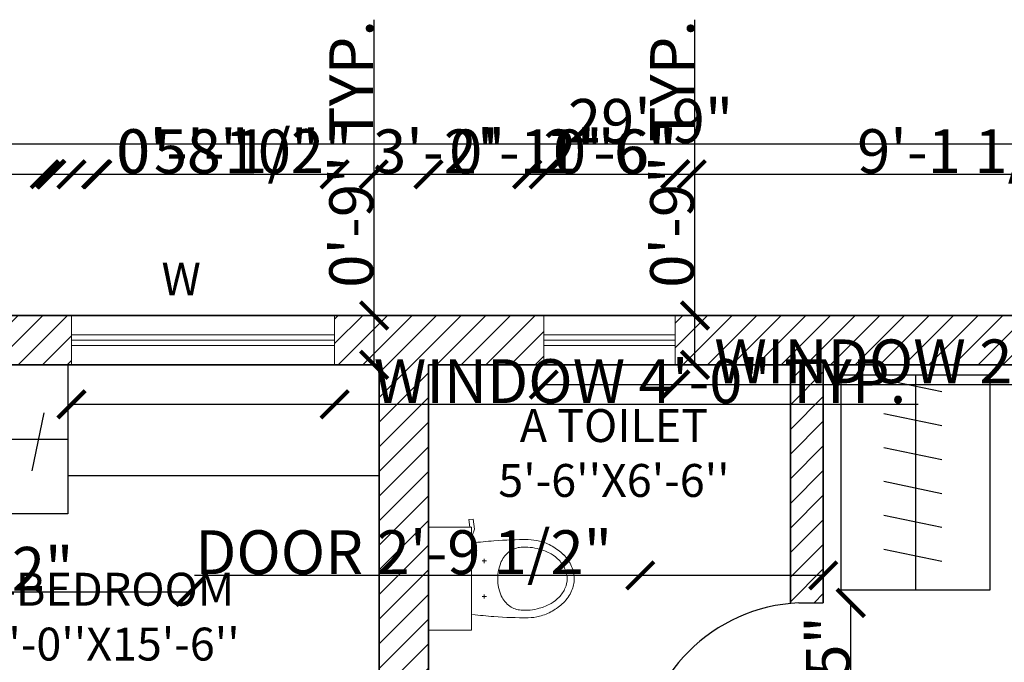
# Model space of a CAD drawing. Units: inches. Extents: x 2094 to 2639, y 1426 to 1997.
# Tile 7 of 8: x 2243 to 2423, y 1866 to 1983. Entities that reach past the tile are written whole.
import ezdxf

# ---------------------------------------------------------------- set-up
doc = ezdxf.new("R2010")
doc.units = ezdxf.units.IN
for name, color, linetype, lineweight in [('A-ANNO-DIMS', 2, 'Continuous', 18), ('A-ANNO-TEXT', 7, 'Continuous', 18), ('A-AREA-IDEN', 7, 'Continuous', 25), ('A-FLOR-CASE', 8, 'Continuous', 25), ('A-FLOR-FIXT', 9, 'Continuous', 18), ('A-WALL-PATT', 8, 'Continuous', 13), ('Doors', 34, 'Continuous', 25), ('Walls', 7, 'Continuous', 35), ('Windows', 150, 'Continuous', 18)]:
    doc.layers.add(name, color=color, linetype=linetype, lineweight=lineweight)
doc.styles.get("Standard").update_dxf_attribs({"font": 'arial.ttf'})
doc.dimstyles.get("Standard").update_dxf_attribs({"dimtxt": 8, "dimasz": 5, "dimexe": 0.18, "dimexo": 0.0625, "dimgap": 0.09, "dimtad": 1, "dimdec": 1, "dimzin": 0, "dimdsep": 46, "dimlunit": 4, "dimtxsty": 'Standard', "dimblk": 'ARCHTICK', "dimcen": 0.09, "dimse1": 1, "dimse2": 1, "dimadec": 0, "dimazin": 0, "dimtfac": 1, "dimtdec": 1, "dimtofl": 0, "dimtmove": 0, "dimatfit": 3, "dimfxl": 1, "dimtolj": 1, "dimtzin": 0, "dimarcsym": 0})

# ---------------------------------------------------------------- blocks, each defined once
blk = doc.blocks.new('AP0B05')
for p, q in [((35, 100), (35, 880)), ((75, 100), (75, 878.9)), ((35, 100), (35, -20)), ((815, 100), (815, -20))]:
    blk.add_line(p, q)
blk.add_lwpolyline([(35, 100), (75, 100)])
blk.add_arc((-2.4, 62.6), 818.3, 2.6212, 87.3788)
blk = doc.blocks.new('toilet-1')
at = {"color": 0, "linetype": 'ByBlock'}
for p, q in [((-0.23, -0.02), (-0.23, -0.2116)), ((0.23, -0.02), (-0.23, -0.02)), ((0.23, -0.02), (0.23, -0.2116)), ((-0.23, -0.2116), (0.23, -0.2116)), ((0.1917, -0.2144), (0.2206, -0.225)), ((0.2206, -0.225), (0.266, -0.2187)), ((0.2633, -0.1997), (0.23, -0.2044)), ((0.266, -0.2187), (0.2633, -0.1997)), ((-0.0793, -0.2587), (-0.0793, -0.2778)), ((0.0794, -0.2587), (0.0794, -0.2778)), ((-0.0889, -0.2683), (-0.0697, -0.2683)), ((0.0889, -0.2683), (0.0698, -0.2683)), ((0, -0.6382), (0, -0.6382))]:
    blk.add_line(p, q, dxfattribs=at)
for centre, radius, start, end in [((3.5272, -0.6239), 3.7093, 173.6925, 175.1593), ((-3.527, -0.624), 3.7093, 4.8413, 6.3171), ((1.7368, -0.4519), 1.9109, 175.7698, 180.3758), ((-0.0312, -0.4465), 0.1114, 113.8997, 145.1485), ((0, -0.5169), 0.1884, 66.0939, 113.9061), ((0.0312, -0.4465), 0.1114, 34.8515, 66.1003), ((-1.7366, -0.4519), 1.9109, 359.6242, 4.2302), ((-0.0408, -0.4398), 0.0996, 145.1497, 175.881), ((0.0409, -0.4398), 0.0996, 4.119, 34.8503), ((0.0981, -0.4497), 0.2389, 175.8862, 195.5931), ((-0.098, -0.4497), 0.2389, 344.4069, 4.1138), ((0.0353, -0.463), 0.2093, 180.3747, 194.3375), ((-0.0351, -0.463), 0.2093, 345.6614, 359.6243), ((0.055, -0.458), 0.2297, 194.3353, 209.622), ((0.0961, -0.4503), 0.2369, 195.5969, 209.3771), ((-0.096, -0.4503), 0.2369, 330.6229, 344.4031), ((-0.0548, -0.458), 0.2297, 330.3788, 345.6655), ((0.0232, -0.4913), 0.1532, 209.3871, 226.5438), ((-0.0231, -0.4913), 0.1532, 313.4562, 330.6129), ((0.0647, -0.4524), 0.2409, 209.6273, 224.5489), ((0.0152, -0.4997), 0.1416, 226.5501, 246.5527), ((-0.0151, -0.4997), 0.1416, 293.4473, 313.4499), ((-0.0645, -0.4524), 0.2409, 315.4504, 330.372), ((0.0178, -0.4986), 0.1751, 224.552, 245.714), ((0.0004, -0.538), 0.132, 245.5845, 269.8782), ((0, -0.5347), 0.1034, 246.5493, 270.0042), ((0, -0.5347), 0.1034, 269.9958, 293.4507), ((-0.0002, -0.538), 0.132, 270.1216, 294.4153), ((-0.0176, -0.4986), 0.1751, 294.2865, 315.4485)]:
    blk.add_arc(centre, radius, start, end, dxfattribs=at)
blk = doc.blocks.new('_ArchTick')
at = {"color": 0, "linetype": 'ByBlock', "const_width": 0.15}
blk.add_lwpolyline([(-0.5, -0.5), (0.5, 0.5)], dxfattribs=at)
blk = doc.blocks.new('*D13')
at = {"layer": 'A-ANNO-DIMS', "color": 0, "lineweight": -2, "transparency": 16777216}
blk.add_line((2180.06, 1960.22), (2537.06, 1960.22), dxfattribs=at)
at = {"layer": 'Defpoints', "color": 0, "transparency": 16777216}
for p in [(2537.06, 1960.22), (2180.06, 1928.9), (2537.06, 1928.9)]:
    blk.add_point(p, dxfattribs=at)
at = {"layer": 'A-ANNO-DIMS', "color": 0, "lineweight": -2, "transparency": 16777216, "xscale": 5, "yscale": 5, "zscale": 5, "rotation": 180}
blk.add_blockref('_ArchTick', (2180.06, 1960.22), dxfattribs=at)
at = {"layer": 'A-ANNO-DIMS', "color": 0, "lineweight": -2, "transparency": 16777216, "xscale": 5, "yscale": 5, "zscale": 5}
blk.add_blockref('_ArchTick', (2537.06, 1960.22), dxfattribs=at)
at = {"layer": 'A-ANNO-DIMS', "color": 0, "transparency": 16777216, "insert": (2358.56, 1964.39), "char_height": 8, "attachment_point": 5}
blk.add_mtext('\\A1;29\'-9"', dxfattribs=at)
blk = doc.blocks.new('WIN-48IN')
for p, q in [((0, 5.5), (48, 5.5)), ((0, 4.5), (48, 4.5)), ((0, 3.5), (48, 3.5))]:
    blk.add_line(p, q)
blk.add_lwpolyline([(0, 0), (48, 0), (48, 9), (0, 9)], close=True)
blk = doc.blocks.new('WIN-24IN')
for p, q in [((24, 5.5), (0, 5.5)), ((24, 4.5), (0, 4.5)), ((24, 3.5), (0, 3.5))]:
    blk.add_line(p, q)
blk.add_lwpolyline([(24, 9), (0, 9), (0, 0), (24, 0)], close=True)
blk = doc.blocks.new('*D19')
at = {"layer": 'A-ANNO-DIMS', "color": 0, "lineweight": -2, "transparency": 16777216}
for p, q in [((2356.68, 1881.5), (2275.36, 1881.5)), ((2390.06, 1881.5), (2356.68, 1881.5))]:
    blk.add_line(p, q, dxfattribs=at)
at = {"layer": 'Defpoints', "color": 0, "transparency": 16777216}
for p in [(2356.68, 1881.5), (2356.68, 1876.49), (2390.06, 1876.49)]:
    blk.add_point(p, dxfattribs=at)
at = {"layer": 'A-ANNO-DIMS', "color": 0, "lineweight": -2, "transparency": 16777216, "xscale": 5, "yscale": 5, "zscale": 5, "rotation": 180}
blk.add_blockref('_ArchTick', (2356.68, 1881.5), dxfattribs=at)
at = {"layer": 'A-ANNO-DIMS', "color": 0, "lineweight": -2, "transparency": 16777216, "xscale": 5, "yscale": 5, "zscale": 5}
blk.add_blockref('_ArchTick', (2390.06, 1881.5), dxfattribs=at)
at = {"layer": 'A-ANNO-DIMS', "color": 0, "transparency": 16777216, "insert": (2313.52, 1885.73), "char_height": 8, "attachment_point": 5}
blk.add_mtext('\\A1;DOOR 2\'-9 1/2"', dxfattribs=at)
blk = doc.blocks.new('*D20')
at = {"layer": 'A-ANNO-DIMS', "color": 0, "lineweight": -2, "transparency": 16777216}
blk.add_line((2395.06, 1847.57), (2395.06, 1876.49), dxfattribs=at)
at = {"layer": 'Defpoints', "color": 0, "transparency": 16777216}
for p in [(2390.06, 1876.49), (2395.06, 1876.49), (2390.06, 1847.57)]:
    blk.add_point(p, dxfattribs=at)
at = {"layer": 'A-ANNO-DIMS', "color": 0, "lineweight": -2, "transparency": 16777216, "xscale": 5, "yscale": 5, "zscale": 5}
for p, rotation in [((2395.06, 1876.49), 90), ((2395.06, 1847.57), 270)]:
    blk.add_blockref('_ArchTick', p, dxfattribs=dict(at, rotation=rotation))
at = {"layer": 'A-ANNO-DIMS', "color": 0, "transparency": 16777216, "insert": (2390.89, 1862.03), "char_height": 8, "attachment_point": 5, "rotation": 90}
blk.add_mtext('\\A1;2\'-5"', dxfattribs=at)
blk = doc.blocks.new('*D27')
at = {"layer": 'A-ANNO-DIMS', "color": 0, "lineweight": -2, "transparency": 16777216}
for p, q in [((2252.94, 1912.7), (2300.94, 1912.7)), ((2300.94, 1912.7), (2407.35, 1912.7))]:
    blk.add_line(p, q, dxfattribs=at)
at = {"layer": 'Defpoints', "color": 0, "transparency": 16777216}
for p in [(2252.94, 1919.9), (2300.94, 1919.9), (2300.94, 1912.7)]:
    blk.add_point(p, dxfattribs=at)
at = {"layer": 'A-ANNO-DIMS', "color": 0, "lineweight": -2, "transparency": 16777216, "xscale": 5, "yscale": 5, "zscale": 5, "rotation": 180}
blk.add_blockref('_ArchTick', (2252.94, 1912.7), dxfattribs=at)
at = {"layer": 'A-ANNO-DIMS', "color": 0, "lineweight": -2, "transparency": 16777216, "xscale": 5, "yscale": 5, "zscale": 5}
blk.add_blockref('_ArchTick', (2300.94, 1912.7), dxfattribs=at)
at = {"layer": 'A-ANNO-DIMS', "color": 0, "transparency": 16777216, "insert": (2356.64, 1916.93), "char_height": 8, "attachment_point": 5}
blk.add_mtext('\\A1;WINDOW 4\'-0" TYP.', dxfattribs=at)
blk = doc.blocks.new('*D28')
at = {"layer": 'A-ANNO-DIMS', "color": 0, "lineweight": -2, "transparency": 16777216}
for p, q in [((2308.14, 1928.9), (2308.14, 1982.84)), ((2308.14, 1919.9), (2308.14, 1928.9))]:
    blk.add_line(p, q, dxfattribs=at)
at = {"layer": 'Defpoints', "color": 0, "transparency": 16777216}
for p in [(2300.94, 1928.9), (2308.14, 1928.9), (2300.94, 1919.9)]:
    blk.add_point(p, dxfattribs=at)
at = {"layer": 'A-ANNO-DIMS', "color": 0, "lineweight": -2, "transparency": 16777216, "xscale": 5, "yscale": 5, "zscale": 5}
for p, rotation in [((2308.14, 1928.9), 90), ((2308.14, 1919.9), 270)]:
    blk.add_blockref('_ArchTick', p, dxfattribs=dict(at, rotation=rotation))
at = {"layer": 'A-ANNO-DIMS', "color": 0, "transparency": 16777216, "insert": (2303.96, 1958.37), "char_height": 8, "attachment_point": 5, "rotation": 90}
blk.add_mtext('\\A1;0\'-9" TYP.', dxfattribs=at)
blk = doc.blocks.new('*D29')
at = {"layer": 'A-ANNO-DIMS', "color": 0, "lineweight": -2, "transparency": 16777216}
for p, q in [((2339.06, 1916.3), (2363.06, 1916.3)), ((2363.06, 1916.3), (2469.47, 1916.3))]:
    blk.add_line(p, q, dxfattribs=at)
at = {"layer": 'Defpoints', "color": 0, "transparency": 16777216}
for p in [(2339.06, 1919.9), (2363.06, 1919.9), (2363.06, 1916.3)]:
    blk.add_point(p, dxfattribs=at)
at = {"layer": 'A-ANNO-DIMS', "color": 0, "lineweight": -2, "transparency": 16777216, "xscale": 5, "yscale": 5, "zscale": 5, "rotation": 180}
blk.add_blockref('_ArchTick', (2339.06, 1916.3), dxfattribs=at)
at = {"layer": 'A-ANNO-DIMS', "color": 0, "lineweight": -2, "transparency": 16777216, "xscale": 5, "yscale": 5, "zscale": 5}
blk.add_blockref('_ArchTick', (2363.06, 1916.3), dxfattribs=at)
at = {"layer": 'A-ANNO-DIMS', "color": 0, "transparency": 16777216, "insert": (2418.76, 1920.53), "char_height": 8, "attachment_point": 5}
blk.add_mtext('\\A1;WINDOW 2\'-0" TYP.', dxfattribs=at)
blk = doc.blocks.new('*D30')
at = {"layer": 'A-ANNO-DIMS', "color": 0, "lineweight": -2, "transparency": 16777216}
for p, q in [((2366.66, 1928.9), (2366.66, 1982.84)), ((2366.66, 1919.9), (2366.66, 1928.9))]:
    blk.add_line(p, q, dxfattribs=at)
at = {"layer": 'Defpoints', "color": 0, "transparency": 16777216}
for p in [(2363.06, 1928.9), (2366.66, 1928.9), (2363.06, 1919.9)]:
    blk.add_point(p, dxfattribs=at)
at = {"layer": 'A-ANNO-DIMS', "color": 0, "lineweight": -2, "transparency": 16777216, "xscale": 5, "yscale": 5, "zscale": 5}
for p, rotation in [((2366.66, 1928.9), 90), ((2366.66, 1919.9), 270)]:
    blk.add_blockref('_ArchTick', p, dxfattribs=dict(at, rotation=rotation))
at = {"layer": 'A-ANNO-DIMS', "color": 0, "transparency": 16777216, "insert": (2362.48, 1958.37), "char_height": 8, "attachment_point": 5, "rotation": 90}
blk.add_mtext('\\A1;0\'-9" TYP.', dxfattribs=at)
blk = doc.blocks.new('*D34')
at = {"layer": 'A-ANNO-DIMS', "color": 0, "lineweight": -2, "transparency": 16777216}
blk.add_line((2274.56, 1878.47), (2189.06, 1878.47), dxfattribs=at)
at = {"layer": 'Defpoints', "color": 0, "transparency": 16777216}
for p in [(2189.06, 1878.47), (2189.06, 1862.67), (2274.56, 1862.67)]:
    blk.add_point(p, dxfattribs=at)
at = {"layer": 'A-ANNO-DIMS', "color": 0, "lineweight": -2, "transparency": 16777216, "xscale": 5, "yscale": 5, "zscale": 5, "rotation": 180}
blk.add_blockref('_ArchTick', (2189.06, 1878.47), dxfattribs=at)
at = {"layer": 'A-ANNO-DIMS', "color": 0, "lineweight": -2, "transparency": 16777216, "xscale": 5, "yscale": 5, "zscale": 5}
blk.add_blockref('_ArchTick', (2274.56, 1878.47), dxfattribs=at)
at = {"layer": 'A-ANNO-DIMS', "color": 0, "transparency": 16777216, "insert": (2231.81, 1882.7), "char_height": 8, "attachment_point": 5}
blk.add_mtext('\\A1;7\'-1 1/2"', dxfattribs=at)
blk = doc.blocks.new('*D53')
at = {"layer": 'A-ANNO-DIMS', "color": 0, "lineweight": -2, "transparency": 16777216}
blk.add_line((2180.06, 1954.65), (2252.94, 1954.65), dxfattribs=at)
at = {"layer": 'Defpoints', "color": 0, "transparency": 16777216}
for p in [(2252.94, 1954.65), (2180.06, 1928.9), (2252.94, 1928.9)]:
    blk.add_point(p, dxfattribs=at)
at = {"layer": 'A-ANNO-DIMS', "color": 0, "lineweight": -2, "transparency": 16777216, "xscale": 5, "yscale": 5, "zscale": 5, "rotation": 180}
blk.add_blockref('_ArchTick', (2180.06, 1954.65), dxfattribs=at)
at = {"layer": 'A-ANNO-DIMS', "color": 0, "lineweight": -2, "transparency": 16777216, "xscale": 5, "yscale": 5, "zscale": 5}
blk.add_blockref('_ArchTick', (2252.94, 1954.65), dxfattribs=at)
at = {"layer": 'A-ANNO-DIMS', "color": 0, "transparency": 16777216, "insert": (2216.5, 1958.82), "char_height": 8, "attachment_point": 5}
blk.add_mtext('\\A1;6\'-1"', dxfattribs=at)
blk = doc.blocks.new('*D54')
at = {"layer": 'A-ANNO-DIMS', "color": 0, "lineweight": -2, "transparency": 16777216}
blk.add_line((2300.94, 1954.65), (2339.06, 1954.65), dxfattribs=at)
at = {"layer": 'Defpoints', "color": 0, "transparency": 16777216}
for p in [(2339.06, 1954.65), (2300.94, 1928.9), (2339.06, 1928.9)]:
    blk.add_point(p, dxfattribs=at)
at = {"layer": 'A-ANNO-DIMS', "color": 0, "lineweight": -2, "transparency": 16777216, "xscale": 5, "yscale": 5, "zscale": 5, "rotation": 180}
blk.add_blockref('_ArchTick', (2300.94, 1954.65), dxfattribs=at)
at = {"layer": 'A-ANNO-DIMS', "color": 0, "lineweight": -2, "transparency": 16777216, "xscale": 5, "yscale": 5, "zscale": 5}
blk.add_blockref('_ArchTick', (2339.06, 1954.65), dxfattribs=at)
at = {"layer": 'A-ANNO-DIMS', "color": 0, "transparency": 16777216, "insert": (2320, 1958.83), "char_height": 8, "attachment_point": 5}
blk.add_mtext('\\A1;3\'-2"', dxfattribs=at)
blk = doc.blocks.new('*D55')
at = {"layer": 'A-ANNO-DIMS', "color": 0, "lineweight": -2, "transparency": 16777216}
blk.add_line((2363.06, 1954.65), (2472.33, 1954.65), dxfattribs=at)
at = {"layer": 'Defpoints', "color": 0, "transparency": 16777216}
for p in [(2472.33, 1954.65), (2363.06, 1928.9), (2472.33, 1928.9)]:
    blk.add_point(p, dxfattribs=at)
at = {"layer": 'A-ANNO-DIMS', "color": 0, "lineweight": -2, "transparency": 16777216, "xscale": 5, "yscale": 5, "zscale": 5, "rotation": 180}
blk.add_blockref('_ArchTick', (2363.06, 1954.65), dxfattribs=at)
at = {"layer": 'A-ANNO-DIMS', "color": 0, "lineweight": -2, "transparency": 16777216, "xscale": 5, "yscale": 5, "zscale": 5}
blk.add_blockref('_ArchTick', (2472.33, 1954.65), dxfattribs=at)
at = {"layer": 'A-ANNO-DIMS', "color": 0, "transparency": 16777216, "insert": (2417.69, 1958.87), "char_height": 8, "attachment_point": 5}
blk.add_mtext('\\A1;9\'-1 1/2"', dxfattribs=at)
blk = doc.blocks.new('*D66')
at = {"layer": 'A-ANNO-DIMS', "color": 0, "lineweight": -2, "transparency": 16777216}
blk.add_line((2336.06, 1954.65), (2366.06, 1954.65), dxfattribs=at)
at = {"layer": 'Defpoints', "color": 0, "transparency": 16777216}
for p in [(2366.06, 1954.65), (2336.06, 1787.9), (2366.06, 1787.9)]:
    blk.add_point(p, dxfattribs=at)
at = {"layer": 'A-ANNO-DIMS', "color": 0, "lineweight": -2, "transparency": 16777216, "xscale": 5, "yscale": 5, "zscale": 5, "rotation": 180}
blk.add_blockref('_ArchTick', (2336.06, 1954.65), dxfattribs=at)
at = {"layer": 'A-ANNO-DIMS', "color": 0, "lineweight": -2, "transparency": 16777216, "xscale": 5, "yscale": 5, "zscale": 5}
blk.add_blockref('_ArchTick', (2366.06, 1954.65), dxfattribs=at)
at = {"layer": 'A-ANNO-DIMS', "color": 0, "transparency": 16777216, "insert": (2351.06, 1958.82), "char_height": 8, "attachment_point": 5}
blk.add_mtext('\\A1;2\'-6"', dxfattribs=at)
blk = doc.blocks.new('*D76')
at = {"layer": 'A-ANNO-DIMS', "color": 0, "lineweight": -2, "transparency": 16777216}
blk.add_line((2248.06, 1954.65), (2318.06, 1954.65), dxfattribs=at)
at = {"layer": 'Defpoints', "color": 0, "transparency": 16777216}
for p in [(2318.06, 1954.65), (2248.06, 1468.9), (2318.06, 1468.9)]:
    blk.add_point(p, dxfattribs=at)
at = {"layer": 'A-ANNO-DIMS', "color": 0, "lineweight": -2, "transparency": 16777216, "xscale": 5, "yscale": 5, "zscale": 5, "rotation": 180}
blk.add_blockref('_ArchTick', (2248.06, 1954.65), dxfattribs=at)
at = {"layer": 'A-ANNO-DIMS', "color": 0, "lineweight": -2, "transparency": 16777216, "xscale": 5, "yscale": 5, "zscale": 5}
blk.add_blockref('_ArchTick', (2318.06, 1954.65), dxfattribs=at)
at = {"layer": 'A-ANNO-DIMS', "color": 0, "transparency": 16777216, "insert": (2283.06, 1958.82), "char_height": 8, "attachment_point": 5}
blk.add_mtext('\\A1;5\'-10"', dxfattribs=at)
blk = doc.blocks.new('*D77')
at = {"layer": 'A-ANNO-DIMS', "color": 0, "lineweight": -2, "transparency": 16777216}
for p, q in [((2308.06, 1954.65), (2318.06, 1954.65)), ((2318.06, 1954.65), (2350.72, 1954.65))]:
    blk.add_line(p, q, dxfattribs=at)
at = {"layer": 'Defpoints', "color": 0, "transparency": 16777216}
for p in [(2318.06, 1954.65), (2308.06, 1468.9), (2318.06, 1468.9)]:
    blk.add_point(p, dxfattribs=at)
at = {"layer": 'A-ANNO-DIMS', "color": 0, "lineweight": -2, "transparency": 16777216, "xscale": 5, "yscale": 5, "zscale": 5, "rotation": 180}
blk.add_blockref('_ArchTick', (2308.06, 1954.65), dxfattribs=at)
at = {"layer": 'A-ANNO-DIMS', "color": 0, "lineweight": -2, "transparency": 16777216, "xscale": 5, "yscale": 5, "zscale": 5}
blk.add_blockref('_ArchTick', (2318.06, 1954.65), dxfattribs=at)
at = {"layer": 'A-ANNO-DIMS', "color": 0, "transparency": 16777216, "insert": (2336.89, 1958.82), "char_height": 8, "attachment_point": 5}
blk.add_mtext('\\A1;0\'-10"', dxfattribs=at)
blk = doc.blocks.new('*D80')
at = {"layer": 'A-ANNO-DIMS', "color": 0, "lineweight": -2, "transparency": 16777216}
for p, q in [((2318.06, 1954.65), (2336.06, 1954.65)), ((2336.06, 1954.65), (2361.75, 1954.65))]:
    blk.add_line(p, q, dxfattribs=at)
at = {"layer": 'Defpoints', "color": 0, "transparency": 16777216}
for p in [(2336.06, 1954.65), (2318.06, 1787.9), (2336.06, 1787.9)]:
    blk.add_point(p, dxfattribs=at)
at = {"layer": 'A-ANNO-DIMS', "color": 0, "lineweight": -2, "transparency": 16777216, "xscale": 5, "yscale": 5, "zscale": 5, "rotation": 180}
blk.add_blockref('_ArchTick', (2318.06, 1954.65), dxfattribs=at)
at = {"layer": 'A-ANNO-DIMS', "color": 0, "lineweight": -2, "transparency": 16777216, "xscale": 5, "yscale": 5, "zscale": 5}
blk.add_blockref('_ArchTick', (2336.06, 1954.65), dxfattribs=at)
at = {"layer": 'A-ANNO-DIMS', "color": 0, "transparency": 16777216, "insert": (2351.4, 1958.82), "char_height": 8, "attachment_point": 5}
blk.add_mtext('\\A1;1\'-6"', dxfattribs=at)
blk = doc.blocks.new('*D81')
at = {"layer": 'A-ANNO-DIMS', "color": 0, "lineweight": -2, "transparency": 16777216}
for p, q in [((2249.13, 1954.65), (2257.66, 1954.65)), ((2257.66, 1954.65), (2302.74, 1954.65))]:
    blk.add_line(p, q, dxfattribs=at)
at = {"layer": 'Defpoints', "color": 0, "transparency": 16777216}
for p in [(2257.66, 1954.65), (2249.13, 1589.48), (2257.66, 1589.48)]:
    blk.add_point(p, dxfattribs=at)
at = {"layer": 'A-ANNO-DIMS', "color": 0, "lineweight": -2, "transparency": 16777216, "xscale": 5, "yscale": 5, "zscale": 5, "rotation": 180}
blk.add_blockref('_ArchTick', (2249.13, 1954.65), dxfattribs=at)
at = {"layer": 'A-ANNO-DIMS', "color": 0, "lineweight": -2, "transparency": 16777216, "xscale": 5, "yscale": 5, "zscale": 5}
blk.add_blockref('_ArchTick', (2257.66, 1954.65), dxfattribs=at)
at = {"layer": 'A-ANNO-DIMS', "color": 0, "transparency": 16777216, "insert": (2282.7, 1958.87), "char_height": 8, "attachment_point": 5}
blk.add_mtext('\\A1;0\'-8 1/2"', dxfattribs=at)
blk = doc.blocks.new('*D83')
at = {"layer": 'A-ANNO-DIMS', "color": 0, "lineweight": -2, "transparency": 16777216}
for p, q in [((2249.25, 1954.65), (2257.43, 1954.65)), ((2257.43, 1954.65), (2283.88, 1954.65))]:
    blk.add_line(p, q, dxfattribs=at)
at = {"layer": 'Defpoints', "color": 0, "transparency": 16777216}
for p in [(2257.43, 1954.65), (2249.25, 1595.79), (2257.43, 1595.79)]:
    blk.add_point(p, dxfattribs=at)
at = {"layer": 'A-ANNO-DIMS', "color": 0, "lineweight": -2, "transparency": 16777216, "xscale": 5, "yscale": 5, "zscale": 5, "rotation": 180}
blk.add_blockref('_ArchTick', (2249.25, 1954.65), dxfattribs=at)
at = {"layer": 'A-ANNO-DIMS', "color": 0, "lineweight": -2, "transparency": 16777216, "xscale": 5, "yscale": 5, "zscale": 5}
blk.add_blockref('_ArchTick', (2257.43, 1954.65), dxfattribs=at)
at = {"layer": 'A-ANNO-DIMS', "color": 0, "transparency": 16777216, "insert": (2273.16, 1958.82), "char_height": 8, "attachment_point": 5}
blk.add_mtext('\\A1;0\'-8"', dxfattribs=at)

msp = doc.modelspace()

# ---------------------------------------------------------------- hatches: boundary and pattern name
at = {"layer": 'A-WALL-PATT', "transparency": 33554585}
h = msp.add_hatch(dxfattribs=at)
h.set_pattern_fill('ANSI31', color=256)
h.paths.add_polyline_path([(2189.06, 1727.9), (2230.3, 1727.9, -0.022928), (2230.09, 1730.2), (2230.09, 1733.9), (2189.06, 1733.9), (2189.06, 1742.37), (2180.06, 1742.37), (2180.06, 1714.4), (2189.06, 1714.4)])
h.paths.add_polyline_path([(2456.51, 1574.9), (2413.83, 1574.9), (2413.83, 1565.9), (2456.51, 1565.9)])
h.paths.add_polyline_path([(2537.06, 1643.81), (2528.06, 1643.81), (2528.06, 1574.9), (2519.78, 1574.9), (2519.78, 1571.88), (2519.78, 1565.9), (2537.06, 1565.9)])
h.paths.add_polyline_path([(2339.06, 1928.9), (2300.94, 1928.9), (2300.94, 1919.9), (2309.06, 1919.9), (2309.06, 1776.3, -0.024186), (2312.62, 1776.64), (2318.06, 1776.64), (2318.06, 1778.9), (2336.06, 1778.9), (2336.06, 1787.9), (2318.06, 1787.9), (2318.06, 1835.9), (2384.06, 1835.9), (2384.06, 1787.9), (2366.06, 1787.9), (2366.06, 1778.9), (2479.64, 1778.9), (2479.64, 1784.88, -0.018603), (2479.89, 1787.9), (2390.06, 1787.9), (2390.06, 1847.57), (2385.61, 1847.57), (2384.06, 1847.57), (2384.06, 1841.9), (2318.06, 1841.9), (2318.06, 1919.9), (2339.06, 1919.9)])
h.paths.add_polyline_path([(2252.94, 1928.9), (2180.06, 1928.9), (2180.06, 1790.37), (2189.06, 1790.37), (2189.06, 1843.77), (2189.06, 1919.9), (2252.94, 1919.9)])
h.paths.add_polyline_path([(2472.33, 1928.9), (2363.06, 1928.9), (2363.06, 1919.9), (2384.06, 1919.9), (2384.06, 1876.38, -0.012802), (2385.61, 1876.49), (2390.06, 1876.49), (2390.06, 1919.9), (2472.33, 1919.9)], flags=17)
h.paths.add_polyline_path([(2537.06, 1928.9), (2520.33, 1928.9), (2520.33, 1919.9), (2528.06, 1919.9), (2528.06, 1905.95), (2528.06, 1787.9), (2518.5, 1787.9), (2518.5, 1784.88), (2518.5, 1778.9), (2528.06, 1778.9), (2528.06, 1715.81), (2537.06, 1715.81)])
h.paths.add_polyline_path([(2379.33, 1857.12), (2393.06, 1857.12), (2393.06, 1866.16), (2379.33, 1866.16)], flags=25)
h.paths.add_polyline_path([(2235.85, 1725.77), (2249.57, 1725.77), (2249.57, 1734.81), (2235.85, 1734.81)], flags=25)
h.paths.add_polyline_path([(2305.79, 1754.6), (2314.84, 1754.6), (2314.84, 1763.6), (2305.79, 1763.6)], flags=9)
h.paths.add_polyline_path([(2493.85, 1778.22), (2502.9, 1778.22), (2502.9, 1787.22), (2493.85, 1787.22)], flags=9)
h.paths.add_polyline_path([(2370.69, 1555.65), (2381.6, 1555.65), (2381.6, 1564.65), (2370.69, 1564.65)], flags=9)
h.paths.add_polyline_path([(2461.57, 1555.65), (2477.6, 1555.65), (2477.6, 1564.65), (2461.57, 1564.65)], flags=9)
h.paths.add_polyline_path([(2493.18, 1565.15), (2509.22, 1565.15), (2509.22, 1574.15), (2493.18, 1574.15)], flags=9)
h.paths.add_polyline_path([(2408.32, 1501.7), (2449.12, 1501.7), (2449.12, 1520.36), (2408.32, 1520.36)], flags=9)
h.paths.add_polyline_path([(2398.49, 1698.6), (2441.61, 1698.6), (2441.61, 1717.26), (2398.49, 1717.26)], flags=9)
h.paths.add_polyline_path([(2248.63, 1683.29), (2287.87, 1683.29), (2287.87, 1701.95), (2248.63, 1701.95)], flags=25)
h.paths.add_polyline_path([(2440.73, 1823.2), (2483.86, 1823.2), (2483.86, 1841.85), (2440.73, 1841.85)], flags=9)
h.paths.add_polyline_path([(2335.3, 1804.5), (2370.65, 1804.5), (2370.65, 1823.15), (2335.3, 1823.15)], flags=25)
h.paths.add_polyline_path([(2335.3, 1893.12), (2370.65, 1893.12), (2370.65, 1911.77), (2335.3, 1911.77)], flags=25)
h.paths.add_polyline_path([(2241.82, 1863.6), (2290.11, 1863.6), (2290.11, 1882.25), (2241.82, 1882.25)], flags=9)

# ---------------------------------------------------------------- linework, layer by layer
at = {"layer": 'A-FLOR-CASE'}
for p, q in [((2406.88, 1918.1), (2406.88, 1878.83)), ((2411.68, 1914.96), (2401.12, 1917.16)), ((2247.88, 1911.13), (2245.68, 1900.57)), ((2411.68, 1908.77), (2401.12, 1910.97)), ((2189.06, 1906.33), (2252.26, 1906.33)), ((2411.68, 1902.58), (2401.12, 1904.78)), ((2252.26, 1899.71), (2309.06, 1899.71)), ((2411.68, 1896.39), (2401.12, 1898.6)), ((2411.68, 1890.21), (2401.12, 1892.41)), ((2411.68, 1884.02), (2401.12, 1886.22))]:
    msp.add_line(p, q, dxfattribs=at)
for points in [[(2189.06, 1919.9), (2252.26, 1919.9), (2252.26, 1892.76), (2189.06, 1892.76)], [(2420.45, 1918.1), (2420.45, 1878.83), (2393.31, 1878.83), (2393.31, 1918.1)]]:
    msp.add_lwpolyline(points, close=True, dxfattribs=at)
at = {"layer": 'Walls'}
for p, q in [((2180.06, 1928.9), (2537.06, 1928.9)), ((2189.06, 1919.9), (2309.06, 1919.9)), ((2309.06, 1919.9), (2309.06, 1776.3)), ((2318.06, 1919.9), (2318.06, 1841.9)), ((2318.06, 1919.9), (2384.06, 1919.9)), ((2384.06, 1919.9), (2384.06, 1876.38)), ((2390.06, 1919.9), (2390.06, 1876.49)), ((2390.06, 1919.9), (2528.06, 1919.9))]:
    msp.add_line(p, q, dxfattribs=at)

# ---------------------------------------------------------------- block references
at = {"layer": 'A-FLOR-FIXT', "xscale": 40.90426662806183, "yscale": 40.90426662806183, "zscale": 40.90426662806183, "rotation": 90}
msp.add_blockref('toilet-1', (2317.24, 1880.9), dxfattribs=at)
at = {"layer": 'Doors', "xscale": 0.0370855999522285, "yscale": 0.0370855999522285, "zscale": 0.0370855999522285, "rotation": 90}
msp.add_blockref('AP0B05', (2389.31, 1846.27), dxfattribs=at)
at = {"layer": 'Windows'}
for name, p in [('WIN-48IN', (2252.94, 1919.9)), ('WIN-24IN', (2339.06, 1919.9))]:
    msp.add_blockref(name, p, dxfattribs=at)

# ---------------------------------------------------------------- texts
at = {"layer": 'A-ANNO-TEXT'}
msp.add_text('W', height=6, dxfattribs=at).set_placement((2269.35, 1932.56))
at = {"layer": 'A-AREA-IDEN', "char_height": 6, "attachment_point": 1}
for s, insert in [("\\pxqc;A TOILET\\P5'-6''X6'-6''", (2325.33, 1911.82)), ("\\pxqc;M-BEDROOM\\P10'-0''X15'-6''", (2231.43, 1881.98))]:
    msp.add_mtext_dynamic_manual_height_columns(s, width=53.0999, gutter_width=63.55, heights=[0], dxfattribs=dict(at, insert=insert))

# ---------------------------------------------------------------- dimensions: what is measured, and where the dimension line sits
at = {"layer": 'A-ANNO-DIMS'}
for base, p1, p2, angle, text, picture, middle in [((2308.14, 1928.9), (2300.94, 1919.9), (2300.94, 1928.9), 90, '<> TYP.', '*D28', (2303.96, 1958.37)), ((2366.66, 1928.9), (2363.06, 1919.9), (2363.06, 1928.9), 90, '<> TYP.', '*D30', (2362.48, 1958.37)), ((2356.68, 1881.5), (2390.06, 1876.49), (2356.68, 1876.49), 180, 'DOOR <>', '*D19', (2313.52, 1885.73))]:
    dim = msp.add_linear_dim(base=base, p1=p1, p2=p2, angle=angle, text=text, dimstyle='Standard', override={"dimdec": 1, "dimlfac": 1, "dimrnd": 0, "dimzin": 1, "dimdsep": 46, "dimlunit": 4, "dimfrac": 2}, dxfattribs=at)
    dim.commit()
    dim.dimension.update_dxf_attribs({"geometry": picture, "text_midpoint": middle})
for base, p1, p2, override, picture, middle in [((2257.66, 1954.65), (2249.13, 1589.48), (2257.66, 1589.48), {"dimdec": 1, "dimlfac": 1, "dimrnd": 0, "dimzin": 1, "dimdsep": 46, "dimlunit": 4, "dimfrac": 2}, '*D81', (2282.7, 1958.87)), ((2472.33, 1954.65), (2363.06, 1928.9), (2472.33, 1928.9), {"dimdec": 1, "dimlfac": 1, "dimrnd": 0, "dimzin": 1, "dimdsep": 46, "dimlunit": 4, "dimfrac": 2}, '*D55', (2417.69, 1958.87)), ((2537.06, 1960.22), (2180.06, 1928.9), (2537.06, 1928.9), {"dimclrd": 0, "dimclre": 0, "dimclrt": 0}, '*D13', (2358.56, 1964.39)), ((2252.94, 1954.65), (2180.06, 1928.9), (2252.94, 1928.9), {"dimdec": 1, "dimlfac": 1, "dimrnd": 0, "dimzin": 1, "dimdsep": 46, "dimlunit": 4, "dimfrac": 2}, '*D53', (2216.5, 1958.82)), ((2318.06, 1954.65), (2248.06, 1468.9), (2318.06, 1468.9), {"dimdec": 1, "dimlfac": 1, "dimrnd": 0, "dimzin": 1, "dimdsep": 46, "dimlunit": 4, "dimfrac": 2}, '*D76', (2283.06, 1958.82)), ((2257.43, 1954.65), (2249.25, 1595.79), (2257.43, 1595.79), {"dimdec": 1, "dimlfac": 1, "dimrnd": 0, "dimzin": 1, "dimdsep": 46, "dimlunit": 4, "dimfrac": 2}, '*D83', (2273.16, 1958.82)), ((2339.06, 1954.65), (2300.94, 1928.9), (2339.06, 1928.9), {"dimdec": 1, "dimlfac": 1, "dimrnd": 0, "dimzin": 1, "dimdsep": 46, "dimlunit": 4, "dimfrac": 2}, '*D54', (2320, 1958.83)), ((2318.06, 1954.65), (2308.06, 1468.9), (2318.06, 1468.9), {"dimdec": 1, "dimlfac": 1, "dimrnd": 0, "dimzin": 1, "dimdsep": 46, "dimlunit": 4, "dimfrac": 2}, '*D77', (2336.89, 1958.82)), ((2336.06, 1954.65), (2318.06, 1787.9), (2336.06, 1787.9), {"dimdec": 1, "dimlfac": 1, "dimrnd": 0, "dimzin": 1, "dimdsep": 46, "dimlunit": 4, "dimfrac": 2}, '*D80', (2351.4, 1958.82)), ((2366.06, 1954.65), (2336.06, 1787.9), (2366.06, 1787.9), {"dimdec": 1, "dimlfac": 1, "dimrnd": 0, "dimzin": 1, "dimdsep": 46, "dimlunit": 4, "dimfrac": 2}, '*D66', (2351.06, 1958.82))]:
    dim = msp.add_linear_dim(base=base, p1=p1, p2=p2, dimstyle='Standard', override=override, dxfattribs=at)
    dim.commit()
    dim.dimension.update_dxf_attribs({"geometry": picture, "text_midpoint": middle})
for base, p1, p2, picture, middle in [((2363.06, 1916.3), (2339.06, 1919.9), (2363.06, 1919.9), '*D29', (2418.76, 1920.53)), ((2300.94, 1912.7), (2252.94, 1919.9), (2300.94, 1919.9), '*D27', (2356.64, 1916.93))]:
    dim = msp.add_linear_dim(base=base, p1=p1, p2=p2, text='WINDOW <> TYP.', dimstyle='Standard', override={"dimdec": 1, "dimlfac": 1, "dimrnd": 0, "dimzin": 1, "dimdsep": 46, "dimlunit": 4, "dimfrac": 2}, dxfattribs=at)
    dim.commit()
    dim.dimension.update_dxf_attribs({"geometry": picture, "text_midpoint": middle})
for base, p1, p2, angle, picture, middle in [((2189.06, 1878.47), (2274.56, 1862.67), (2189.06, 1862.67), 180, '*D34', (2231.81, 1882.7)), ((2395.06, 1876.49), (2390.06, 1847.57), (2390.06, 1876.49), 90, '*D20', (2390.89, 1862.03))]:
    dim = msp.add_linear_dim(base=base, p1=p1, p2=p2, angle=angle, dimstyle='Standard', override={"dimdec": 1, "dimlfac": 1, "dimrnd": 0, "dimzin": 1, "dimdsep": 46, "dimlunit": 4, "dimfrac": 2}, dxfattribs=at)
    dim.commit()
    dim.dimension.update_dxf_attribs({"geometry": picture, "text_midpoint": middle})

doc.saveas('drawing.dxf')
